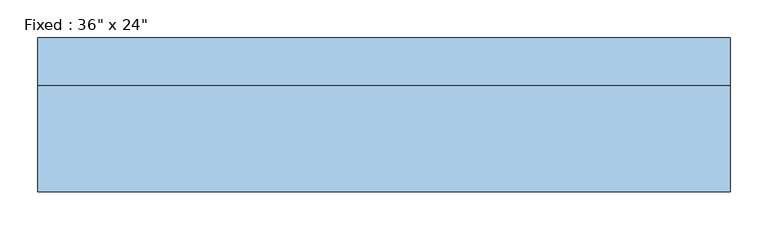
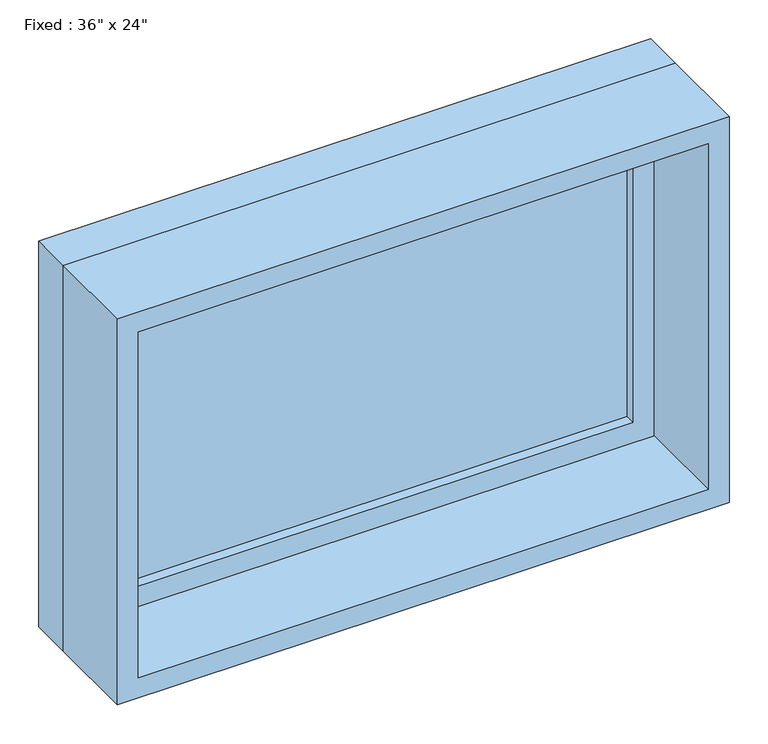
"""IFC4 building model written with IfcOpenShell, lengths in millimetres: window geometry."""

from ifc_helpers import new_model, si_unit, frame, origin, place, context, project, spatial, polyline, outline, extrude, source, transform, mapped, element, save


def window_57c3ee1c(model_context):
    return source(origin(), model_context, "Body", "SweptSolid", [
        extrude(outline(polyline([(355.6, 53.975), (-431.8, 53.975), (-431.8, 66.675), (355.6, 66.675), (355.6, 53.975)])), frame((0.0, 0.0, 977.9), z_axis=(0.0, 0.0, 1.0), x_axis=(1.0, 0.0, 0.0)), (0.0, 0.0, 1.0), 482.6),
        extrude(outline(polyline([(1504.95, -476.25), (933.45, -476.25), (933.45, 400.05), (1504.95, 400.05), (1504.95, -476.25)]), holes=[polyline([(1460.5, -431.8), (1460.5, 355.6), (977.9, 355.6), (977.9, -431.8), (1460.5, -431.8)])]), frame((0.0, 38.1, 0.0), z_axis=(0.0, 1.0, 0.0), x_axis=(0.0, 0.0, 1.0)), (0.0, 0.0, 1.0), 44.45),
        extrude(outline(polyline([(1524.0, -495.3), (914.4, -495.3), (914.4, 419.1), (1524.0, 419.1), (1524.0, -495.3)]), holes=[polyline([(1492.25, -463.55), (1492.25, 387.35), (946.15, 387.35), (946.15, -463.55), (1492.25, -463.55)])]), frame((0.0, -101.6, 0.0), z_axis=(0.0, 1.0, 0.0), x_axis=(0.0, 0.0, 1.0)), (0.0, 0.0, 1.0), 139.7),
        extrude(outline(polyline([(1524.0, 419.1), (1524.0, -495.3), (914.4, -495.3), (914.4, 419.1), (1524.0, 419.1)]), holes=[polyline([(1504.95, 400.05), (933.45, 400.05), (933.45, -476.25), (1504.95, -476.25), (1504.95, 400.05)])]), frame((0.0, 38.1, 0.0), z_axis=(0.0, 1.0, 0.0), x_axis=(0.0, 0.0, 1.0)), (0.0, 0.0, 1.0), 63.5),
    ])


if __name__ == "__main__":
    model = new_model("IFC4")
    model_context = context("Model", 3, world=origin())
    ifc_project = project(units=[si_unit("LENGTHUNIT", "METRE", prefix="MILLI")], contexts=[model_context])
    site = spatial("IfcSite", under=ifc_project)
    building = spatial("IfcBuilding", under=site)
    placement = place(None, origin())
    window_shape = window_57c3ee1c(model_context)
    element("IfcWindow", 1, ObjectType="Fixed : 36\" x 24\"", at=placement, inside=building, context=model_context, shape_type="MappedRepresentation", body=[
        mapped(window_shape, transform((0.0, 0.0, 0.0), x_axis=(1.0, 0.0, 0.0), y_axis=(0.0, 1.0, 0.0), z_axis=(0.0, 0.0, 1.0))),
    ])
    save(model, "model.ifc")

# Revit data of these elements
# Type "Fixed : 36\" x 24\""
#   Type Mark = "8"
#   Construction Type Id = "GSP4R"
#   Assembly Code = "B2020100"
#   Analytic Construction = "1/8 in Pilkington single glazing"
#   Visual Light Transmittance = 0.9
#   Solar Heat Gain Coefficient = 0.78
#   Heat Transfer Coefficient (U) = 0.6496 BTU/(h·ft²·°F)
#   Height = 2' - 0"
#   Default Sill Height = 3' - 0"
#   Width = 3' - 0"
#   Window Inset = 0' - 0 3/4"
#   Define Thermal Properties by = 1
#   Glass Pane Material = Glass
#   Sash Material = Sash
#   Wall Closure = (empty or 0)
# Element 1 (IfcWindow, "Fixed : 36\" x 24\"")
#   Materials on its faces: "Sash", "Glass"
# Materials
#   "Glass": class "Glass", colour RGB 0 128 192, transparency 0.75, Description = "Soda Lime Glass", Cost = 0
#   "Sash": class "Wood", colour RGB 224 178 126, transparency 0
